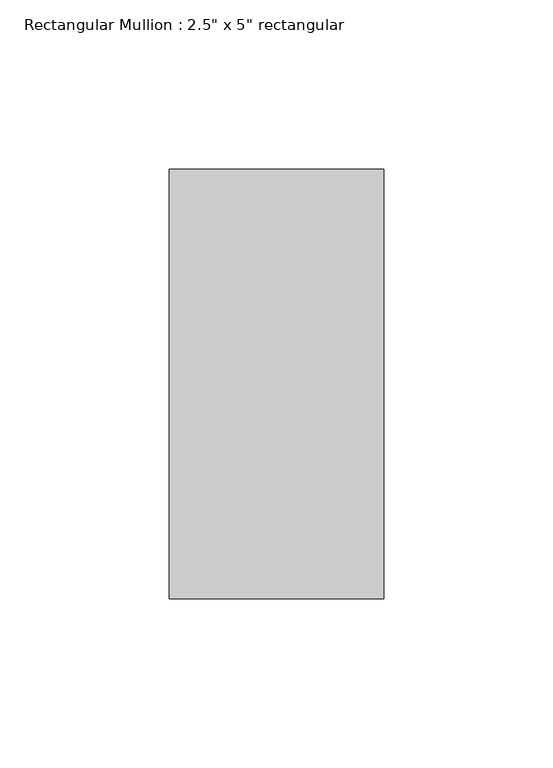
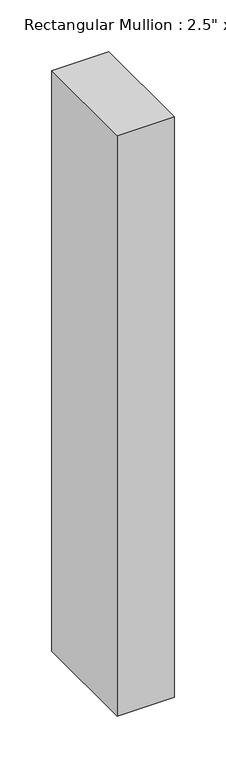
"""IFC4 building model written with IfcOpenShell, lengths in millimetres: member geometry."""

from ifc_helpers import new_model, si_unit, frame, origin, place, context, project, spatial, polyline, outline, extrude, source, transform, mapped, element, save


def member_892f3d40(model_context):
    return source(origin(), model_context, "Body", "SweptSolid", [
        extrude(outline(polyline([(0.0, 63.5), (0.0, -63.5), (-63.5, -63.5), (-63.5, 63.5), (0.0, 63.5)])), frame((0.0, 0.0, -685.4574877), z_axis=(0.0, 0.0, 1.0), x_axis=(1.0, 0.0, 0.0)), (0.0, 0.0, 1.0), 685.4574877),
    ])


if __name__ == "__main__":
    model = new_model("IFC4")
    model_context = context("Model", 3, world=origin())
    ifc_project = project(units=[si_unit("LENGTHUNIT", "METRE", prefix="MILLI")], contexts=[model_context])
    site = spatial("IfcSite", under=ifc_project)
    building = spatial("IfcBuilding", under=site)
    placement = place(None, origin())
    member_shape = member_892f3d40(model_context)
    element("IfcMember", 1, ObjectType="Rectangular Mullion : 2.5\" x 5\" rectangular", at=placement, inside=building, context=model_context, shape_type="MappedRepresentation", body=[
        mapped(member_shape, transform((0.0, 0.0, 0.0), x_axis=(1.0, 0.0, 0.0), y_axis=(0.0, 1.0, 0.0), z_axis=(0.0, 0.0, 1.0))),
    ])
    save(model, "model.ifc")

# Revit data of these elements
# Type "Rectangular Mullion : 2.5\" x 5\" rectangular"
#   built-in parameter 1007304 = 0.416667 (stored number, unit not read)
#   built-in parameter 1007301 = 0.104167 (stored number, unit not read)
#   built-in parameter 1007300 = 0.104167 (stored number, unit not read)
# Element 1 (IfcMember, "Rectangular Mullion : 2.5\" x 5\" rectangular")
#   Materials on its faces: "Aluminum"
# Materials
#   "Aluminum": class "Metal", colour RGB 247 247 247, transparency 0, Description = "Aluminum 6061", Cost = 0
